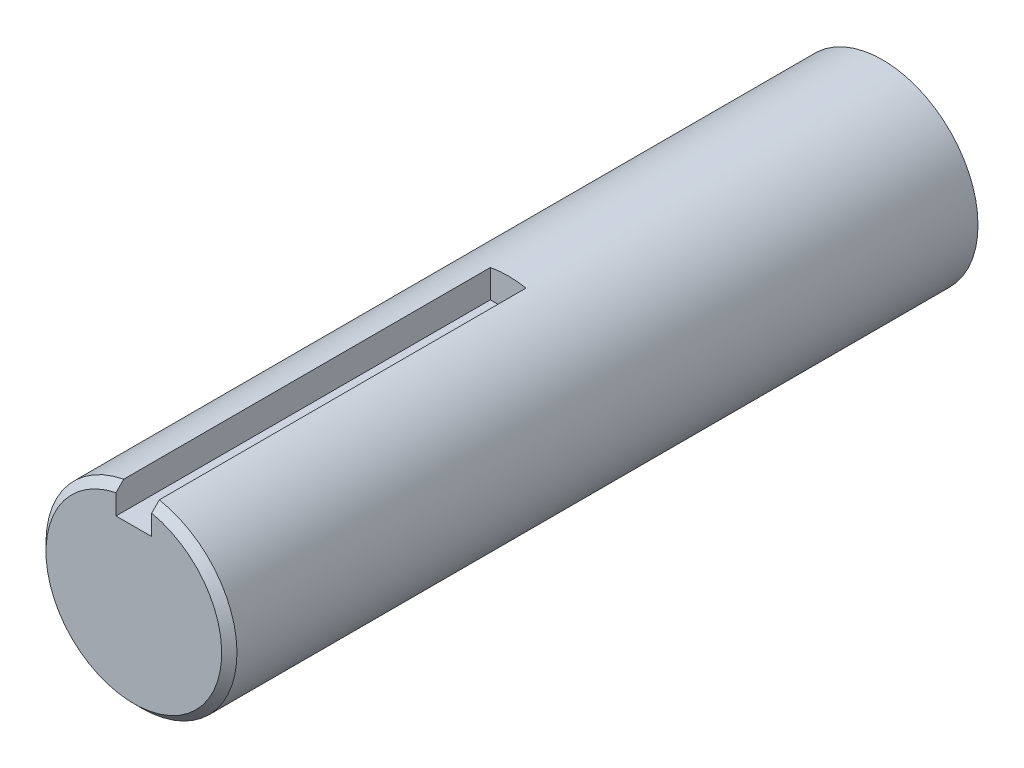
ISO-10303-21;
HEADER;
FILE_DESCRIPTION(('STEP AP214'),'2;1');
FILE_NAME('part.step','',(''),(''),'','','');
FILE_SCHEMA(('AUTOMOTIVE_DESIGN { 1 0 10303 214 1 1 1 1 }'));
ENDSEC;
DATA;
#1=APPLICATION_CONTEXT('core data for automotive mechanical design processes');
#2=APPLICATION_PROTOCOL_DEFINITION('international standard','automotive_design',2000,#1);
#3=PRODUCT_CONTEXT('',#1,'mechanical');
#4=PRODUCT('Part','Part','',(#3));
#5=PRODUCT_RELATED_PRODUCT_CATEGORY('part','',(#4));
#6=PRODUCT_DEFINITION_FORMATION('','',#4);
#7=PRODUCT_DEFINITION_CONTEXT('part definition',#1,'design');
#8=PRODUCT_DEFINITION('design','',#6,#7);
#9=PRODUCT_DEFINITION_SHAPE('','',#8);
#10=(LENGTH_UNIT() NAMED_UNIT(*) SI_UNIT(.MILLI.,.METRE.));
#11=(NAMED_UNIT(*) PLANE_ANGLE_UNIT() SI_UNIT($,.RADIAN.));
#12=(NAMED_UNIT(*) SI_UNIT($,.STERADIAN.) SOLID_ANGLE_UNIT());
#13=UNCERTAINTY_MEASURE_WITH_UNIT(LENGTH_MEASURE(1.E-05),#10,'distance_accuracy_value','');
#14=(GEOMETRIC_REPRESENTATION_CONTEXT(3) GLOBAL_UNCERTAINTY_ASSIGNED_CONTEXT((#13)) GLOBAL_UNIT_ASSIGNED_CONTEXT((#10,
#11,#12)) REPRESENTATION_CONTEXT('',''));
#15=CARTESIAN_POINT('',(0.,0.,0.));
#16=DIRECTION('',(0.,0.,1.));
#17=DIRECTION('',(1.,0.,0.));
#18=AXIS2_PLACEMENT_3D('',#15,#16,#17);
#19=CARTESIAN_POINT('',(0.,0.,294.));
#20=DIRECTION('',(0.,0.,-1.));
#21=DIRECTION('',(-1.,0.,0.));
#22=AXIS2_PLACEMENT_3D('',#19,#20,#21);
#23=CYLINDRICAL_SURFACE('',#22,37.5);
#24=DIRECTION('',(0.,0.,1.));
#25=VECTOR('',#24,1.);
#26=CARTESIAN_POINT('',(7.,36.8408740395773,147.));
#27=LINE('',#26,#25);
#28=CARTESIAN_POINT('',(7.,36.8408740395773,147.));
#29=VERTEX_POINT('',#28);
#30=CARTESIAN_POINT('',(7.,36.8408740395773,291.));
#31=VERTEX_POINT('',#30);
#32=EDGE_CURVE('E127',#29,#31,#27,.T.);
#33=ORIENTED_EDGE('',*,*,#32,.T.);
#34=CARTESIAN_POINT('',(0.,0.,291.));
#35=DIRECTION('',(0.,0.,1.));
#36=DIRECTION('',(1.,0.,0.));
#37=AXIS2_PLACEMENT_3D('',#34,#35,#36);
#38=CIRCLE('',#37,37.5);
#39=CARTESIAN_POINT('',(-7.,36.8408740395773,291.));
#40=VERTEX_POINT('',#39);
#41=EDGE_CURVE('E59',#31,#40,#38,.F.);
#42=ORIENTED_EDGE('',*,*,#41,.T.);
#43=DIRECTION('',(0.,0.,1.));
#44=VECTOR('',#43,1.);
#45=CARTESIAN_POINT('',(-7.,36.8408740395773,147.));
#46=LINE('',#45,#44);
#47=CARTESIAN_POINT('',(-7.,36.8408740395773,147.));
#48=VERTEX_POINT('',#47);
#49=EDGE_CURVE('E98',#48,#40,#46,.T.);
#50=ORIENTED_EDGE('',*,*,#49,.F.);
#51=CARTESIAN_POINT('',(0.,0.,147.));
#52=DIRECTION('',(0.,0.,1.));
#53=DIRECTION('',(1.,0.,0.));
#54=AXIS2_PLACEMENT_3D('',#51,#52,#53);
#55=CIRCLE('',#54,37.5);
#56=EDGE_CURVE('E106',#29,#48,#55,.T.);
#57=ORIENTED_EDGE('',*,*,#56,.F.);
#58=EDGE_LOOP('',(#33,#42,#50,#57));
#59=FACE_BOUND('',#58,.T.);
#60=CARTESIAN_POINT('',(0.,0.,0.));
#61=DIRECTION('',(0.,0.,1.));
#62=DIRECTION('',(1.,0.,0.));
#63=AXIS2_PLACEMENT_3D('',#60,#61,#62);
#64=CIRCLE('',#63,37.5);
#65=CARTESIAN_POINT('',(37.5,0.,0.));
#66=VERTEX_POINT('',#65);
#67=EDGE_CURVE('E125',#66,#66,#64,.T.);
#68=ORIENTED_EDGE('',*,*,#67,.T.);
#69=EDGE_LOOP('',(#68));
#70=FACE_BOUND('',#69,.T.);
#71=ADVANCED_FACE('F43',(#59,#70),#23,.T.);
#72=CARTESIAN_POINT('',(0.,0.,294.));
#73=DIRECTION('',(0.,0.,1.));
#74=DIRECTION('',(1.,0.,0.));
#75=AXIS2_PLACEMENT_3D('',#72,#73,#74);
#76=PLANE('',#75);
#77=DIRECTION('',(0.,-1.,0.));
#78=VECTOR('',#77,1.);
#79=CARTESIAN_POINT('',(-7.,25.8408740395773,294.));
#80=LINE('',#79,#78);
#81=CARTESIAN_POINT('',(-7.,33.7823918632177,294.));
#82=VERTEX_POINT('',#81);
#83=CARTESIAN_POINT('',(-7.,25.8408740395773,294.));
#84=VERTEX_POINT('',#83);
#85=EDGE_CURVE('E206',#82,#84,#80,.T.);
#86=ORIENTED_EDGE('',*,*,#85,.F.);
#87=CARTESIAN_POINT('',(0.,0.,294.));
#88=DIRECTION('',(0.,0.,1.));
#89=DIRECTION('',(1.,0.,0.));
#90=AXIS2_PLACEMENT_3D('',#87,#88,#89);
#91=CIRCLE('',#90,34.5);
#92=CARTESIAN_POINT('',(7.,33.7823918632177,294.));
#93=VERTEX_POINT('',#92);
#94=EDGE_CURVE('E124',#82,#93,#91,.T.);
#95=ORIENTED_EDGE('',*,*,#94,.T.);
#96=DIRECTION('',(0.,1.,0.));
#97=VECTOR('',#96,1.);
#98=CARTESIAN_POINT('',(7.,25.8408740395773,294.));
#99=LINE('',#98,#97);
#100=CARTESIAN_POINT('',(7.,25.8408740395773,294.));
#101=VERTEX_POINT('',#100);
#102=EDGE_CURVE('E114',#101,#93,#99,.T.);
#103=ORIENTED_EDGE('',*,*,#102,.F.);
#104=DIRECTION('',(1.,0.,0.));
#105=VECTOR('',#104,1.);
#106=CARTESIAN_POINT('',(-7.,25.8408740395773,294.));
#107=LINE('',#106,#105);
#108=EDGE_CURVE('E209',#84,#101,#107,.T.);
#109=ORIENTED_EDGE('',*,*,#108,.F.);
#110=EDGE_LOOP('',(#86,#95,#103,#109));
#111=FACE_BOUND('',#110,.T.);
#112=ADVANCED_FACE('F148',(#111),#76,.T.);
#113=CARTESIAN_POINT('',(0.,0.,0.));
#114=DIRECTION('',(0.,0.,1.));
#115=DIRECTION('',(1.,0.,0.));
#116=AXIS2_PLACEMENT_3D('',#113,#114,#115);
#117=PLANE('',#116);
#118=ORIENTED_EDGE('',*,*,#67,.F.);
#119=EDGE_LOOP('',(#118));
#120=FACE_BOUND('',#119,.T.);
#121=ADVANCED_FACE('F139',(#120),#117,.F.);
#122=CARTESIAN_POINT('',(7.,25.8408740395773,147.));
#123=DIRECTION('',(1.,0.,0.));
#124=DIRECTION('',(0.,0.,-1.));
#125=AXIS2_PLACEMENT_3D('',#122,#123,#124);
#126=PLANE('',#125);
#127=ORIENTED_EDGE('',*,*,#102,.T.);
#128=CARTESIAN_POINT('',(7.,33.7823918632177,294.));
#129=CARTESIAN_POINT('',(7.,34.2925489046528,293.500417997698));
#130=CARTESIAN_POINT('',(7.,34.8025009418508,293.000626994794));
#131=CARTESIAN_POINT('',(7.,35.8219950006316,292.000626994789));
#132=CARTESIAN_POINT('',(7.,36.3315370222201,291.500417997692));
#133=CARTESIAN_POINT('',(7.,36.8408740395773,291.));
#134=B_SPLINE_CURVE_WITH_KNOTS('',3,(#128,#129,#130,#131,#132,#133),.UNSPECIFIED.,.F.,.F.,(4,2,
4),(0.,2.14209690290434,4.28419377579915),.UNSPECIFIED.);
#135=EDGE_CURVE('E75',#93,#31,#134,.T.);
#136=ORIENTED_EDGE('',*,*,#135,.T.);
#137=ORIENTED_EDGE('',*,*,#32,.F.);
#138=DIRECTION('',(0.,1.,0.));
#139=VECTOR('',#138,1.);
#140=CARTESIAN_POINT('',(7.,25.8408740395773,147.));
#141=LINE('',#140,#139);
#142=CARTESIAN_POINT('',(7.,25.8408740395773,147.));
#143=VERTEX_POINT('',#142);
#144=EDGE_CURVE('E115',#143,#29,#141,.T.);
#145=ORIENTED_EDGE('',*,*,#144,.F.);
#146=DIRECTION('',(0.,0.,1.));
#147=VECTOR('',#146,1.);
#148=CARTESIAN_POINT('',(7.,25.8408740395773,147.));
#149=LINE('',#148,#147);
#150=EDGE_CURVE('E120',#143,#101,#149,.T.);
#151=ORIENTED_EDGE('',*,*,#150,.T.);
#152=EDGE_LOOP('',(#127,#136,#137,#145,#151));
#153=FACE_BOUND('',#152,.T.);
#154=ADVANCED_FACE('F133',(#153),#126,.F.);
#155=CARTESIAN_POINT('',(-7.,25.8408740395773,147.));
#156=DIRECTION('',(0.,-1.,0.));
#157=DIRECTION('',(0.,0.,-1.));
#158=AXIS2_PLACEMENT_3D('',#155,#156,#157);
#159=PLANE('',#158);
#160=ORIENTED_EDGE('',*,*,#108,.T.);
#161=ORIENTED_EDGE('',*,*,#150,.F.);
#162=DIRECTION('',(1.,0.,0.));
#163=VECTOR('',#162,1.);
#164=CARTESIAN_POINT('',(-7.,25.8408740395773,147.));
#165=LINE('',#164,#163);
#166=CARTESIAN_POINT('',(-7.,25.8408740395773,147.));
#167=VERTEX_POINT('',#166);
#168=EDGE_CURVE('E104',#167,#143,#165,.T.);
#169=ORIENTED_EDGE('',*,*,#168,.F.);
#170=DIRECTION('',(0.,0.,1.));
#171=VECTOR('',#170,1.);
#172=CARTESIAN_POINT('',(-7.,25.8408740395773,147.));
#173=LINE('',#172,#171);
#174=EDGE_CURVE('E101',#167,#84,#173,.T.);
#175=ORIENTED_EDGE('',*,*,#174,.T.);
#176=EDGE_LOOP('',(#160,#161,#169,#175));
#177=FACE_BOUND('',#176,.T.);
#178=ADVANCED_FACE('F137',(#177),#159,.F.);
#179=CARTESIAN_POINT('',(-7.,25.8408740395773,147.));
#180=DIRECTION('',(-1.,0.,0.));
#181=DIRECTION('',(0.,0.,1.));
#182=AXIS2_PLACEMENT_3D('',#179,#180,#181);
#183=PLANE('',#182);
#184=ORIENTED_EDGE('',*,*,#49,.T.);
#185=CARTESIAN_POINT('',(-7.,36.8408740395773,291.));
#186=CARTESIAN_POINT('',(-7.,36.3315370222201,291.500417997692));
#187=CARTESIAN_POINT('',(-7.,35.8219950006316,292.000626994789));
#188=CARTESIAN_POINT('',(-7.,34.8025009418508,293.000626994794));
#189=CARTESIAN_POINT('',(-7.,34.2925489046528,293.500417997698));
#190=CARTESIAN_POINT('',(-7.,33.7823918632177,294.));
#191=B_SPLINE_CURVE_WITH_KNOTS('',3,(#185,#186,#187,#188,#189,#190),.UNSPECIFIED.,.F.,.F.,(4,2,
4),(0.,2.14209687289482,4.28419377579915),.UNSPECIFIED.);
#192=EDGE_CURVE('E11',#40,#82,#191,.T.);
#193=ORIENTED_EDGE('',*,*,#192,.T.);
#194=ORIENTED_EDGE('',*,*,#85,.T.);
#195=ORIENTED_EDGE('',*,*,#174,.F.);
#196=DIRECTION('',(0.,-1.,0.));
#197=VECTOR('',#196,1.);
#198=CARTESIAN_POINT('',(-7.,25.8408740395773,147.));
#199=LINE('',#198,#197);
#200=EDGE_CURVE('E92',#48,#167,#199,.T.);
#201=ORIENTED_EDGE('',*,*,#200,.F.);
#202=EDGE_LOOP('',(#184,#193,#194,#195,#201));
#203=FACE_BOUND('',#202,.T.);
#204=ADVANCED_FACE('F100',(#203),#183,.F.);
#205=CARTESIAN_POINT('',(0.,0.,147.));
#206=DIRECTION('',(0.,0.,1.));
#207=DIRECTION('',(1.,0.,0.));
#208=AXIS2_PLACEMENT_3D('',#205,#206,#207);
#209=PLANE('',#208);
#210=ORIENTED_EDGE('',*,*,#56,.T.);
#211=ORIENTED_EDGE('',*,*,#200,.T.);
#212=ORIENTED_EDGE('',*,*,#168,.T.);
#213=ORIENTED_EDGE('',*,*,#144,.T.);
#214=EDGE_LOOP('',(#210,#211,#212,#213));
#215=FACE_BOUND('',#214,.T.);
#216=ADVANCED_FACE('F109',(#215),#209,.T.);
#217=CARTESIAN_POINT('',(0.,0.,294.));
#218=DIRECTION('',(0.,0.,-1.));
#219=DIRECTION('',(-1.,0.,0.));
#220=AXIS2_PLACEMENT_3D('',#217,#218,#219);
#221=CONICAL_SURFACE('',#220,34.5,0.785398163397458);
#222=ORIENTED_EDGE('',*,*,#192,.F.);
#223=ORIENTED_EDGE('',*,*,#41,.F.);
#224=ORIENTED_EDGE('',*,*,#135,.F.);
#225=ORIENTED_EDGE('',*,*,#94,.F.);
#226=EDGE_LOOP('',(#222,#223,#224,#225));
#227=FACE_BOUND('',#226,.T.);
#228=ADVANCED_FACE('F46',(#227),#221,.T.);
#229=CLOSED_SHELL('',(#71,#112,#121,#154,#178,#204,#216,#228));
#230=MANIFOLD_SOLID_BREP('B2',#229);
#231=ADVANCED_BREP_SHAPE_REPRESENTATION('',(#18,#230),#14);
#232=SHAPE_DEFINITION_REPRESENTATION(#9,#231);
ENDSEC;
END-ISO-10303-21;
